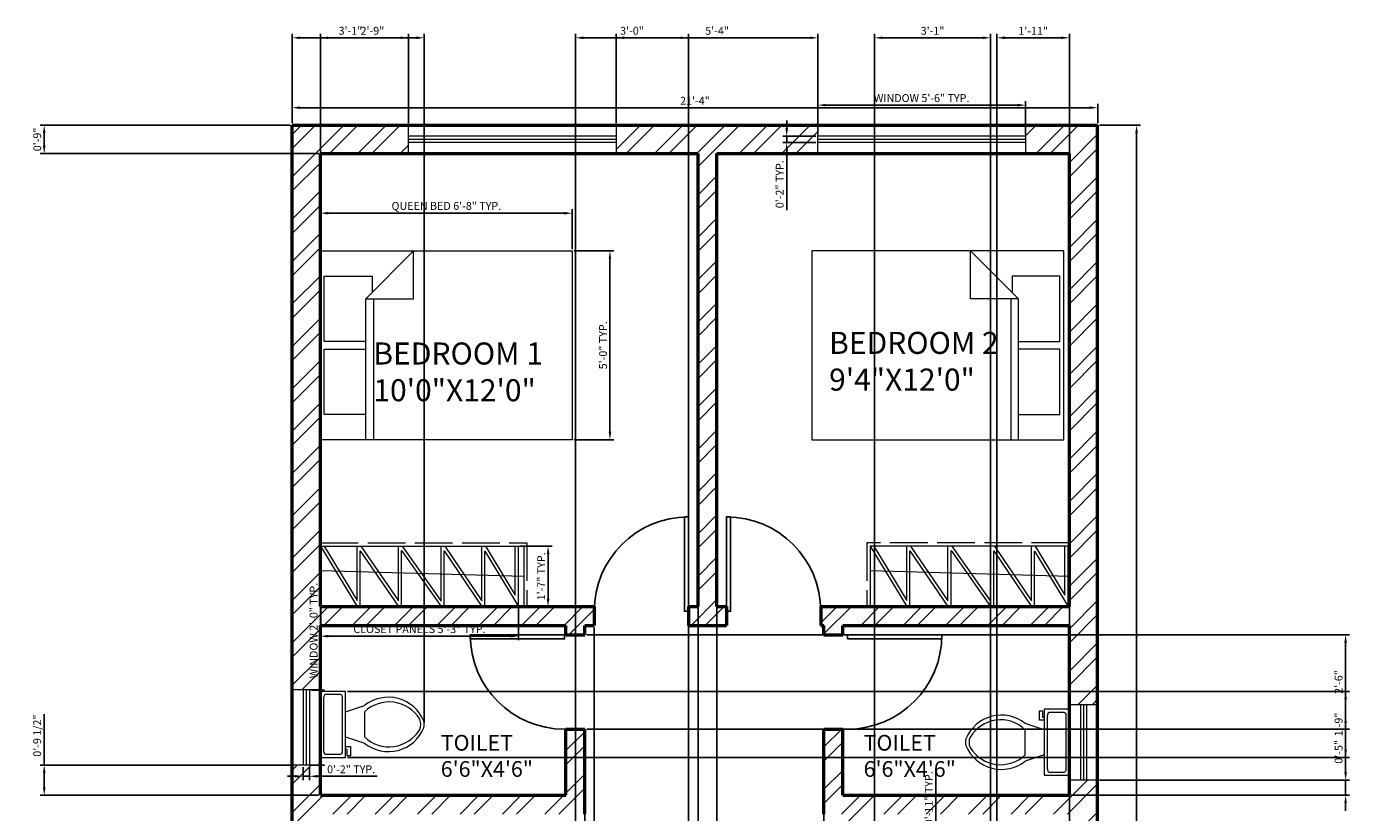
# Model space of a CAD drawing. Units: inches. Extents: x 1147 to 1568, y 1982 to 2559.
# Tile 4 of 4: x 1147 to 1568, y 2309 to 2559. Entities that reach past the tile are written whole.
import ezdxf

# ---------------------------------------------------------------- set-up
doc = ezdxf.new("R2010")
doc.units = ezdxf.units.IN
doc.linetypes.add('ACAD_ISO02W100', pattern=[15, 12, -3])
for name, color, linetype, lineweight in [('A-ANNO-DIMS', 2, 'Continuous', 18), ('A-DOOR', 4, 'Continuous', 25), ('A-FLOR-CASE', 8, 'Continuous', 18), ('A-FLOR-CASE-HIDN', 8, 'ACAD_ISO02W100', 18), ('A-FLOR-FIXT', 8, 'Continuous', 18), ('A-WALL', 7, 'Continuous', 50), ('A-WALL-PATT', 252, 'Continuous', 13)]:
    doc.layers.add(name, color=color, linetype=linetype, lineweight=lineweight)
for name, color, linetype, lineweight, true_color in [('A-AREA-IDEN', 244, 'Continuous', 25, 0x991b1e), ('A-FURN', 244, 'Continuous', 18, 0x991b1e), ('A-GLAZ', 177, 'Continuous', 18, 0x293189)]:
    doc.layers.add(name, color=color, linetype=linetype, lineweight=lineweight, true_color=true_color)
doc.styles.get("Standard").update_dxf_attribs({"font": 'arial.ttf'})
doc.dimstyles.new('ISO-25', dxfattribs={"dimtxt": 2.5, "dimasz": 2.5, "dimexe": 1.25, "dimexo": 0.625, "dimtad": 1, "dimlunit": 3, "dimtxsty": 'Standard', "dimcen": 2.5, "dimadec": 0, "dimazin": 0, "dimtfac": 1, "dimtmove": 0, "dimatfit": 3, "dimfxl": 1, "dimarcsym": 0})

# ---------------------------------------------------------------- blocks, each defined once
blk = doc.blocks.new('*U2')
for p, q in [((0, 0), (0, -6)), ((-40, 0), (-40, -6))]:
    blk.add_line(p, q)
blk.add_lwpolyline([(0, 0), (0, 40), (-1.75, 40), (-1.75, 0)], close=True)
blk.add_arc((0, 0), 40, 90, 180)
blk = doc.blocks.new('*U3')
for p, q in [((-40, 0), (-40, 6)), ((0, 0), (0, 6))]:
    blk.add_line(p, q)
blk.add_lwpolyline([(0, 0), (0, -40), (-1.75, -40), (-1.75, 0)], close=True)
blk.add_arc((0, 0), 40, 180, 270)
blk = doc.blocks.new('Bed - Queen')
for p, q in [((0, -80.00003), (0, 0)), ((0, 0), (59.99999, 0)), ((59.99999, 0), (59.99999, -80.00003)), ((7.99999, -1.2), (28.79998, -1.2)), ((7.99999, -14.4), (7.99999, -1.2)), ((28.79998, -1.2), (28.79998, -14.4)), ((31.19999, -1.2), (51.99999, -1.2)), ((31.19999, -14.4), (31.19999, -1.2)), ((51.99999, -1.2), (51.99999, -16.4)), ((0, -14.4), (44.8, -14.4)), ((44.8, -16.8), (0, -16.8)), ((59.99999, -29.6), (44.8, -14.4)), ((44.8, -14.4), (44.8, -29.6)), ((51.99999, -16.4), (46.79936, -16.4)), ((44.8, -29.6), (59.99999, -29.6)), ((59.99999, -80.00003), (0, -80.00003))]:
    blk.add_line(p, q)
blk = doc.blocks.new('*U6')
for p, q in [((9.5, -6), (9.5, -2)), ((-8, -8.5), (-8, -8)), ((-7, -8), (-7, -9.5)), ((-4, -8), (-6, -14)), ((4, -8), (6, -14)), ((-10, -8.5), (-8, -8.5)), ((-10, -9.5), (-10, -8.5)), ((-7, -9.5), (-10, -9.5)), ((4, -14), (-4, -14))]:
    blk.add_line(p, q)
blk.add_lwpolyline([(10.5, -8), (10.5, 0), (-10.5, 0), (-10.5, -8)], close=True)
for points in [[(-9.5, -2), (-9.5, -6)], [(8.5, -1), (-8.5, -1)], [(-8.5, -7), (8.5, -7)]]:
    blk.add_lwpolyline(points)
for centre, radius, start, end in [((-8.62, -1.88), 0.884, 81.8699, 188.1301), ((8.62, -1.88), 0.884, 351.8699, 98.1301), ((-8.62, -6.12), 0.884, 171.8699, 278.1301), ((8.62, -6.12), 0.884, 261.8699, 8.1301), ((3.52, -21.58), 12.17, 141.4691, 247.9714), ((4.2, -21.82), 11.33, 136.3677, 238.9468), ((-3.52, -21.58), 12.17, 292.0284, 38.5307), ((-4.2, -21.82), 11.33, 301.053, 43.6321), ((0, -27.88), 4, 245.7318, 294.2682), ((0, -29), 4, 254.8605, 285.1395)]:
    blk.add_arc(centre, radius, start, end)
blk = doc.blocks.new('*D13')
at = {"layer": 'A-ANNO-DIMS', "color": 0, "lineweight": -2, "transparency": 16777216}
for p, q in [((1488.23, 2527.7), (1501.22, 2527.7)), ((1499.97, 2525.2), (1499.97, 2020.2)), ((1488.23, 2017.7), (1501.22, 2017.7))]:
    blk.add_line(p, q, dxfattribs=at)
at = {"layer": 'A-ANNO-DIMS', "color": 0, "transparency": 16777216}
for points in [[(1499.56, 2525.2), (1500.39, 2525.2), (1499.97, 2527.7)], [(1499.56, 2020.2), (1500.39, 2020.2), (1499.97, 2017.7)]]:
    blk.add_solid(points, dxfattribs=at)
at = {"layer": 'Defpoints', "color": 0, "transparency": 16777216}
for p in [(1487.61, 2527.7), (1487.61, 2017.7), (1499.97, 2017.7)]:
    blk.add_point(p, dxfattribs=at)
at = {"layer": 'A-ANNO-DIMS', "color": 0, "transparency": 16777216, "insert": (1498.07, 2272.7), "char_height": 2.5, "attachment_point": 5, "rotation": 90}
blk.add_mtext('42\'-6"', dxfattribs=at)
blk = doc.blocks.new('*D14')
at = {"layer": 'A-ANNO-DIMS', "color": 0, "lineweight": -2, "transparency": 16777216}
for p, q in [((1231.61, 2528.33), (1231.61, 2534.54)), ((1485.11, 2533.29), (1234.11, 2533.29)), ((1487.61, 2528.33), (1487.61, 2534.54))]:
    blk.add_line(p, q, dxfattribs=at)
at = {"layer": 'A-ANNO-DIMS', "color": 0, "transparency": 16777216}
for points in [[(1234.11, 2533.7), (1234.11, 2532.87), (1231.61, 2533.29)], [(1485.11, 2533.7), (1485.11, 2532.87), (1487.61, 2533.29)]]:
    blk.add_solid(points, dxfattribs=at)
at = {"layer": 'Defpoints', "color": 0, "transparency": 16777216}
for p in [(1231.61, 2533.29), (1231.61, 2527.7), (1487.61, 2527.7)]:
    blk.add_point(p, dxfattribs=at)
at = {"layer": 'A-ANNO-DIMS', "color": 0, "transparency": 16777216, "insert": (1359.61, 2535.17), "char_height": 2.5, "attachment_point": 5}
blk.add_mtext('21\'-4"', dxfattribs=at)
blk = doc.blocks.new('WIN-GLAZ-66IN')
for p, q in [((0, 2), (66, 2)), ((0, 1), (66, 1)), ((0, 0), (66, 0))]:
    blk.add_line(p, q)
blk = doc.blocks.new('WIN-GLAZ-24IN')
for p, q in [((0, 23.82), (0, 0)), ((1, 23.82), (1, 0)), ((2, 23.82), (2, 0))]:
    blk.add_line(p, q)
blk = doc.blocks.new('CLOSET-PANEL-SET')
for p, q in [((0, 19.2), (11.64, 0)), ((1.17, 19.2), (11.64, 1.93)), ((11.64, 1.93), (11.64, 19.2)), ((12.64, 17.74), (24.75, 0)), ((12.64, 0), (12.64, 17.74)), ((12.85, 19.2), (24.75, 1.77)), ((24.75, 1.77), (24.75, 19.2)), ((25.75, 17.78), (38.31, 0)), ((25.75, 0), (25.75, 17.78)), ((25.98, 19.2), (38.31, 1.73)), ((38.31, 1.73), (38.31, 19.2)), ((39.31, 17.72), (51.27, 0)), ((39.31, 0), (39.31, 17.72)), ((39.52, 19.2), (51.27, 1.79)), ((51.27, 1.79), (51.27, 19.2)), ((52.27, 17.55), (62.9, 0)), ((52.27, 0), (52.27, 17.55)), ((52.44, 19.2), (61.9, 3.58)), ((61.9, 3.58), (61.9, 19.2)), ((62.9, 0), (62.9, 19.2))]:
    blk.add_line(p, q)
blk = doc.blocks.new('*D21')
at = {"layer": 'A-ANNO-DIMS', "color": 0, "lineweight": -2, "transparency": 16777216}
for p, q in [((1398.68, 2524.83), (1398.68, 2535.35)), ((1462.18, 2534.1), (1401.18, 2534.1)), ((1464.68, 2524.83), (1464.68, 2535.35))]:
    blk.add_line(p, q, dxfattribs=at)
at = {"layer": 'A-ANNO-DIMS', "color": 0, "transparency": 16777216}
for points in [[(1401.18, 2534.52), (1401.18, 2533.69), (1398.68, 2534.1)], [(1462.18, 2534.52), (1462.18, 2533.69), (1464.68, 2534.1)]]:
    blk.add_solid(points, dxfattribs=at)
at = {"layer": 'Defpoints', "color": 0, "transparency": 16777216}
for p in [(1398.68, 2534.1), (1398.68, 2524.2), (1464.68, 2524.2)]:
    blk.add_point(p, dxfattribs=at)
at = {"layer": 'A-ANNO-DIMS', "color": 0, "transparency": 16777216, "insert": (1431.68, 2536.02), "char_height": 2.5, "attachment_point": 5}
blk.add_mtext('WINDOW 5\'-6" TYP.', dxfattribs=at)
blk = doc.blocks.new('*D22')
at = {"layer": 'A-ANNO-DIMS', "color": 0, "lineweight": -2, "transparency": 16777216}
for p, q in [((1388.78, 2526.7), (1388.78, 2529.2)), ((1398.05, 2524.2), (1387.53, 2524.2)), ((1388.78, 2524.2), (1388.78, 2522.2)), ((1398.05, 2522.2), (1387.53, 2522.2)), ((1388.78, 2519.7), (1388.78, 2500.72))]:
    blk.add_line(p, q, dxfattribs=at)
at = {"layer": 'A-ANNO-DIMS', "color": 0, "transparency": 16777216}
for points in [[(1388.36, 2526.7), (1389.2, 2526.7), (1388.78, 2524.2)], [(1388.36, 2519.7), (1389.2, 2519.7), (1388.78, 2522.2)]]:
    blk.add_solid(points, dxfattribs=at)
at = {"layer": 'Defpoints', "color": 0, "transparency": 16777216}
for p in [(1398.68, 2524.2), (1388.78, 2522.2), (1398.68, 2522.2)]:
    blk.add_point(p, dxfattribs=at)
at = {"layer": 'A-ANNO-DIMS', "color": 0, "transparency": 16777216, "insert": (1386.88, 2508.96), "char_height": 2.5, "attachment_point": 5, "rotation": 90}
blk.add_mtext('0\'-2" TYP.', dxfattribs=at)
blk = doc.blocks.new('*D23')
at = {"layer": 'A-ANNO-DIMS', "color": 0, "lineweight": -2, "transparency": 16777216}
for p, q in [((1240.68, 2348.11), (1240.68, 2383.5)), ((1237.73, 2348.11), (1241.93, 2348.11)), ((1240.68, 2326.8), (1240.68, 2345.61)), ((1237.73, 2324.3), (1241.93, 2324.3))]:
    blk.add_line(p, q, dxfattribs=at)
at = {"layer": 'A-ANNO-DIMS', "color": 0, "transparency": 16777216}
for points in [[(1240.26, 2345.61), (1241.1, 2345.61), (1240.68, 2348.11)], [(1240.26, 2326.8), (1241.1, 2326.8), (1240.68, 2324.3)]]:
    blk.add_solid(points, dxfattribs=at)
at = {"layer": 'Defpoints', "color": 0, "transparency": 16777216}
for p in [(1237.11, 2348.11), (1240.68, 2348.11), (1237.11, 2324.3)]:
    blk.add_point(p, dxfattribs=at)
at = {"layer": 'A-ANNO-DIMS', "color": 0, "transparency": 16777216, "insert": (1238.76, 2367.06), "char_height": 2.5, "attachment_point": 5, "rotation": 90}
blk.add_mtext('WINDOW 2\'-0" TYP.', dxfattribs=at)
blk = doc.blocks.new('*D24')
at = {"layer": 'A-ANNO-DIMS', "color": 0, "lineweight": -2, "transparency": 16777216}
for p, q in [((1235.11, 2323.67), (1235.11, 2319.47)), ((1237.11, 2323.67), (1237.11, 2319.47)), ((1232.61, 2320.72), (1230.11, 2320.72)), ((1235.11, 2320.72), (1237.11, 2320.72)), ((1239.61, 2320.72), (1258.6, 2320.72))]:
    blk.add_line(p, q, dxfattribs=at)
at = {"layer": 'A-ANNO-DIMS', "color": 0, "transparency": 16777216}
for points in [[(1232.61, 2321.14), (1232.61, 2320.31), (1235.11, 2320.72)], [(1239.61, 2321.14), (1239.61, 2320.31), (1237.11, 2320.72)]]:
    blk.add_solid(points, dxfattribs=at)
at = {"layer": 'Defpoints', "color": 0, "transparency": 16777216}
for p in [(1235.11, 2324.3), (1237.11, 2324.3), (1237.11, 2320.72)]:
    blk.add_point(p, dxfattribs=at)
at = {"layer": 'A-ANNO-DIMS', "color": 0, "transparency": 16777216, "insert": (1250.35, 2322.62), "char_height": 2.5, "attachment_point": 5}
blk.add_mtext('0\'-2" TYP.', dxfattribs=at)
blk = doc.blocks.new('*D27')
at = {"layer": 'A-ANNO-DIMS', "color": 0, "lineweight": -2, "transparency": 16777216}
for p, q in [((1240.61, 2488.36), (1240.61, 2500.99)), ((1318.11, 2499.74), (1243.11, 2499.74)), ((1320.61, 2488.36), (1320.61, 2500.99))]:
    blk.add_line(p, q, dxfattribs=at)
at = {"layer": 'A-ANNO-DIMS', "color": 0, "transparency": 16777216}
for points in [[(1243.11, 2500.16), (1243.11, 2499.32), (1240.61, 2499.74)], [(1318.11, 2500.16), (1318.11, 2499.32), (1320.61, 2499.74)]]:
    blk.add_solid(points, dxfattribs=at)
at = {"layer": 'Defpoints', "color": 0, "transparency": 16777216}
for p in [(1240.61, 2499.74), (1240.61, 2487.74), (1320.61, 2487.74)]:
    blk.add_point(p, dxfattribs=at)
at = {"layer": 'A-ANNO-DIMS', "color": 0, "transparency": 16777216, "insert": (1280.61, 2501.73), "char_height": 2.5, "attachment_point": 5}
blk.add_mtext('QUEEN BED 6\'-8" TYP.', dxfattribs=at)
blk = doc.blocks.new('*D28')
at = {"layer": 'A-ANNO-DIMS', "color": 0, "lineweight": -2, "transparency": 16777216}
for p, q in [((1321.23, 2487.74), (1333.86, 2487.74)), ((1332.61, 2430.24), (1332.61, 2485.24)), ((1321.23, 2427.74), (1333.86, 2427.74))]:
    blk.add_line(p, q, dxfattribs=at)
at = {"layer": 'A-ANNO-DIMS', "color": 0, "transparency": 16777216}
for points in [[(1332.19, 2485.24), (1333.02, 2485.24), (1332.61, 2487.74)], [(1332.19, 2430.24), (1333.02, 2430.24), (1332.61, 2427.74)]]:
    blk.add_solid(points, dxfattribs=at)
at = {"layer": 'Defpoints', "color": 0, "transparency": 16777216}
for p in [(1320.61, 2487.74), (1332.61, 2487.74), (1320.61, 2427.74)]:
    blk.add_point(p, dxfattribs=at)
at = {"layer": 'A-ANNO-DIMS', "color": 0, "transparency": 16777216, "insert": (1330.71, 2457.74), "char_height": 2.5, "attachment_point": 5, "rotation": 90}
blk.add_mtext('5\'-0" TYP.', dxfattribs=at)
blk = doc.blocks.new('*D32')
at = {"layer": 'A-ANNO-DIMS', "color": 0, "lineweight": -2, "transparency": 16777216}
for p, q in [((1436.16, 2302.04), (1436.16, 2322.97)), ((1434.67, 2302.04), (1437.41, 2302.04)), ((1436.16, 2293.51), (1436.16, 2299.54)), ((1434.67, 2291.01), (1437.41, 2291.01))]:
    blk.add_line(p, q, dxfattribs=at)
at = {"layer": 'A-ANNO-DIMS', "color": 0, "transparency": 16777216}
for points in [[(1435.75, 2299.54), (1436.58, 2299.54), (1436.16, 2302.04)], [(1435.75, 2293.51), (1436.58, 2293.51), (1436.16, 2291.01)]]:
    blk.add_solid(points, dxfattribs=at)
at = {"layer": 'Defpoints', "color": 0, "transparency": 16777216}
for p in [(1434.04, 2302.04), (1436.16, 2302.04), (1434.04, 2291.01)]:
    blk.add_point(p, dxfattribs=at)
at = {"layer": 'A-ANNO-DIMS', "color": 0, "transparency": 16777216, "insert": (1434.26, 2313.75), "char_height": 2.5, "attachment_point": 5, "rotation": 90}
blk.add_mtext('0\'-11" TYP.', dxfattribs=at)
blk = doc.blocks.new('*D33')
at = {"layer": 'A-ANNO-DIMS', "color": 0, "lineweight": -2, "transparency": 16777216}
for p, q in [((1240.61, 2374.08), (1240.61, 2364.02)), ((1303.5, 2374.08), (1303.5, 2364.02)), ((1243.11, 2365.27), (1301, 2365.27))]:
    blk.add_line(p, q, dxfattribs=at)
at = {"layer": 'A-ANNO-DIMS', "color": 0, "transparency": 16777216}
for points in [[(1243.11, 2365.69), (1243.11, 2364.85), (1240.61, 2365.27)], [(1301, 2365.69), (1301, 2364.85), (1303.5, 2365.27)]]:
    blk.add_solid(points, dxfattribs=at)
at = {"layer": 'Defpoints', "color": 0, "transparency": 16777216}
for p in [(1240.61, 2374.7), (1303.5, 2374.7), (1303.5, 2365.27)]:
    blk.add_point(p, dxfattribs=at)
at = {"layer": 'A-ANNO-DIMS', "color": 0, "transparency": 16777216, "insert": (1272.06, 2367.19), "char_height": 2.5, "attachment_point": 5}
blk.add_mtext('CLOSET PANELS 5\'-3" TYP.', dxfattribs=at)
blk = doc.blocks.new('*D34')
at = {"layer": 'A-ANNO-DIMS', "color": 0, "lineweight": -2, "transparency": 16777216}
for p, q in [((1304.13, 2393.9), (1314.19, 2393.9)), ((1312.94, 2377.2), (1312.94, 2391.4)), ((1304.13, 2374.7), (1314.19, 2374.7))]:
    blk.add_line(p, q, dxfattribs=at)
at = {"layer": 'A-ANNO-DIMS', "color": 0, "transparency": 16777216}
for points in [[(1312.52, 2391.4), (1313.36, 2391.4), (1312.94, 2393.9)], [(1312.52, 2377.2), (1313.36, 2377.2), (1312.94, 2374.7)]]:
    blk.add_solid(points, dxfattribs=at)
at = {"layer": 'Defpoints', "color": 0, "transparency": 16777216}
for p in [(1303.5, 2393.9), (1312.94, 2393.9), (1303.5, 2374.7)]:
    blk.add_point(p, dxfattribs=at)
at = {"layer": 'A-ANNO-DIMS', "color": 0, "transparency": 16777216, "insert": (1311.06, 2384.3), "char_height": 2.5, "attachment_point": 5, "rotation": 90}
blk.add_mtext('1\'-7" TYP.', dxfattribs=at)
blk = doc.blocks.new('*D43')
at = {"layer": 'A-ANNO-DIMS', "color": 0, "lineweight": -2, "transparency": 16777216}
for p, q in [((1327.61, 2368.08), (1327.61, 1981.52)), ((1357.61, 2368.08), (1357.61, 1981.52)), ((1330.11, 1982.77), (1355.11, 1982.77))]:
    blk.add_line(p, q, dxfattribs=at)
at = {"layer": 'A-ANNO-DIMS', "color": 0, "transparency": 16777216}
for points in [[(1330.11, 1983.19), (1330.11, 1982.35), (1327.61, 1982.77)], [(1355.11, 1983.19), (1355.11, 1982.35), (1357.61, 1982.77)]]:
    blk.add_solid(points, dxfattribs=at)
at = {"layer": 'Defpoints', "color": 0, "transparency": 16777216}
for p in [(1327.61, 2368.7), (1357.61, 2368.7), (1357.61, 1982.77)]:
    blk.add_point(p, dxfattribs=at)
at = {"layer": 'A-ANNO-DIMS', "color": 0, "transparency": 16777216, "insert": (1342.61, 1984.67), "char_height": 2.5, "attachment_point": 5}
blk.add_mtext('2\'-6"', dxfattribs=at)
blk = doc.blocks.new('*D44')
at = {"layer": 'A-ANNO-DIMS', "color": 0, "lineweight": -2, "transparency": 16777216}
for p, q in [((1325.23, 2365.7), (1567.66, 2365.7)), ((1566.41, 2338.2), (1566.41, 2363.2)), ((1325.23, 2335.7), (1567.66, 2335.7))]:
    blk.add_line(p, q, dxfattribs=at)
at = {"layer": 'A-ANNO-DIMS', "color": 0, "transparency": 16777216}
for points in [[(1565.99, 2363.2), (1566.82, 2363.2), (1566.41, 2365.7)], [(1565.99, 2338.2), (1566.82, 2338.2), (1566.41, 2335.7)]]:
    blk.add_solid(points, dxfattribs=at)
at = {"layer": 'Defpoints', "color": 0, "transparency": 16777216}
for p in [(1324.61, 2365.7), (1566.41, 2365.7), (1324.61, 2335.7)]:
    blk.add_point(p, dxfattribs=at)
at = {"layer": 'A-ANNO-DIMS', "color": 0, "transparency": 16777216, "insert": (1564.51, 2350.7), "char_height": 2.5, "attachment_point": 5, "rotation": 90}
blk.add_mtext('2\'-6"', dxfattribs=at)
blk = doc.blocks.new('*D45')
at = {"layer": 'A-ANNO-DIMS', "color": 0, "lineweight": -2, "transparency": 16777216}
for p, q in [((1321.61, 2177.33), (1321.61, 2556.75)), ((1357.61, 2177.33), (1357.61, 2556.75)), ((1324.11, 2555.5), (1355.11, 2555.5))]:
    blk.add_line(p, q, dxfattribs=at)
at = {"layer": 'A-ANNO-DIMS', "color": 0, "transparency": 16777216}
for points in [[(1324.11, 2555.92), (1324.11, 2555.09), (1321.61, 2555.5)], [(1355.11, 2555.92), (1355.11, 2555.09), (1357.61, 2555.5)]]:
    blk.add_solid(points, dxfattribs=at)
at = {"layer": 'Defpoints', "color": 0, "transparency": 16777216}
for p in [(1357.61, 2555.5), (1321.61, 2176.7), (1357.61, 2176.7)]:
    blk.add_point(p, dxfattribs=at)
at = {"layer": 'A-ANNO-DIMS', "color": 0, "transparency": 16777216, "insert": (1339.61, 2557.41), "char_height": 2.5, "attachment_point": 5}
blk.add_mtext('3\'-0"', dxfattribs=at)
blk = doc.blocks.new('*D51')
at = {"layer": 'A-ANNO-DIMS', "color": 0, "lineweight": -2, "transparency": 16777216}
for p, q in [((1360.61, 2518.08), (1360.61, 1981.52)), ((1366.61, 2518.08), (1366.61, 1981.52)), ((1358.11, 1982.77), (1355.61, 1982.77)), ((1360.61, 1982.77), (1366.61, 1982.77)), ((1369.11, 1982.77), (1379.5, 1982.77))]:
    blk.add_line(p, q, dxfattribs=at)
at = {"layer": 'A-ANNO-DIMS', "color": 0, "transparency": 16777216}
for points in [[(1358.11, 1983.19), (1358.11, 1982.35), (1360.61, 1982.77)], [(1369.11, 1983.19), (1369.11, 1982.35), (1366.61, 1982.77)]]:
    blk.add_solid(points, dxfattribs=at)
at = {"layer": 'Defpoints', "color": 0, "transparency": 16777216}
for p in [(1360.61, 2518.7), (1366.61, 2518.7), (1366.61, 1982.77)]:
    blk.add_point(p, dxfattribs=at)
at = {"layer": 'A-ANNO-DIMS', "color": 0, "transparency": 16777216, "insert": (1375.55, 1984.67), "char_height": 2.5, "attachment_point": 5}
blk.add_mtext('0\'-6"', dxfattribs=at)
blk = doc.blocks.new('*D52')
at = {"layer": 'A-ANNO-DIMS', "color": 0, "lineweight": -2, "transparency": 16777216}
for p, q in [((1231.61, 2528.33), (1231.61, 2556.75)), ((1268.63, 2528.33), (1268.63, 2556.75)), ((1234.11, 2555.5), (1266.13, 2555.5))]:
    blk.add_line(p, q, dxfattribs=at)
at = {"layer": 'A-ANNO-DIMS', "color": 0, "transparency": 16777216}
for points in [[(1234.11, 2555.92), (1234.11, 2555.09), (1231.61, 2555.5)], [(1266.13, 2555.92), (1266.13, 2555.09), (1268.63, 2555.5)]]:
    blk.add_solid(points, dxfattribs=at)
at = {"layer": 'Defpoints', "color": 0, "transparency": 16777216}
for p in [(1268.63, 2555.5), (1231.61, 2527.7), (1268.63, 2527.7)]:
    blk.add_point(p, dxfattribs=at)
at = {"layer": 'A-ANNO-DIMS', "color": 0, "transparency": 16777216, "insert": (1250.12, 2557.41), "char_height": 2.5, "attachment_point": 5}
blk.add_mtext('3\'-1"', dxfattribs=at)
blk = doc.blocks.new('*D53')
at = {"layer": 'A-ANNO-DIMS', "color": 0, "lineweight": -2, "transparency": 16777216}
for p, q in [((1334.63, 2528.33), (1334.63, 2556.75)), ((1398.68, 2528.33), (1398.68, 2556.75)), ((1337.13, 2555.5), (1396.18, 2555.5))]:
    blk.add_line(p, q, dxfattribs=at)
at = {"layer": 'A-ANNO-DIMS', "color": 0, "transparency": 16777216}
for points in [[(1337.13, 2555.92), (1337.13, 2555.09), (1334.63, 2555.5)], [(1396.18, 2555.92), (1396.18, 2555.09), (1398.68, 2555.5)]]:
    blk.add_solid(points, dxfattribs=at)
at = {"layer": 'Defpoints', "color": 0, "transparency": 16777216}
for p in [(1398.68, 2555.5), (1334.63, 2527.7), (1398.68, 2527.7)]:
    blk.add_point(p, dxfattribs=at)
at = {"layer": 'A-ANNO-DIMS', "color": 0, "transparency": 16777216, "insert": (1366.65, 2557.4), "char_height": 2.5, "attachment_point": 5}
blk.add_mtext('5\'-4"', dxfattribs=at)
blk = doc.blocks.new('*D54')
at = {"layer": 'A-ANNO-DIMS', "color": 0, "lineweight": -2, "transparency": 16777216}
for p, q in [((1230.98, 2527.7), (1151.56, 2527.7)), ((1152.81, 2525.2), (1152.81, 2521.2)), ((1239.98, 2518.7), (1151.56, 2518.7))]:
    blk.add_line(p, q, dxfattribs=at)
at = {"layer": 'A-ANNO-DIMS', "color": 0, "transparency": 16777216}
for points in [[(1152.39, 2525.2), (1153.22, 2525.2), (1152.81, 2527.7)], [(1152.39, 2521.2), (1153.22, 2521.2), (1152.81, 2518.7)]]:
    blk.add_solid(points, dxfattribs=at)
at = {"layer": 'Defpoints', "color": 0, "transparency": 16777216}
for p in [(1231.61, 2527.7), (1152.81, 2518.7), (1240.61, 2518.7)]:
    blk.add_point(p, dxfattribs=at)
at = {"layer": 'A-ANNO-DIMS', "color": 0, "transparency": 16777216, "insert": (1150.91, 2523.2), "char_height": 2.5, "attachment_point": 5, "rotation": 90}
blk.add_mtext('0\'-9"', dxfattribs=at)
blk = doc.blocks.new('*D58')
at = {"layer": 'A-ANNO-DIMS', "color": 0, "lineweight": -2, "transparency": 16777216}
for p, q in [((1152.81, 2324.3), (1152.81, 2340.52)), ((1230.98, 2324.3), (1151.56, 2324.3)), ((1152.81, 2317.2), (1152.81, 2321.8)), ((1239.98, 2314.7), (1151.56, 2314.7))]:
    blk.add_line(p, q, dxfattribs=at)
at = {"layer": 'A-ANNO-DIMS', "color": 0, "transparency": 16777216}
for points in [[(1152.39, 2321.8), (1153.22, 2321.8), (1152.81, 2324.3)], [(1152.39, 2317.2), (1153.22, 2317.2), (1152.81, 2314.7)]]:
    blk.add_solid(points, dxfattribs=at)
at = {"layer": 'Defpoints', "color": 0, "transparency": 16777216}
for p in [(1152.81, 2324.3), (1231.61, 2324.3), (1240.61, 2314.7)]:
    blk.add_point(p, dxfattribs=at)
at = {"layer": 'A-ANNO-DIMS', "color": 0, "transparency": 16777216, "insert": (1150.89, 2333.66), "char_height": 2.5, "attachment_point": 5, "rotation": 90}
blk.add_mtext('0\'-9 1/2"', dxfattribs=at)
blk = doc.blocks.new('*D59')
at = {"layer": 'A-ANNO-DIMS', "color": 0, "lineweight": -2, "transparency": 16777216}
for p, q in [((1566.41, 2322.05), (1566.41, 2332.44)), ((1488.23, 2319.55), (1567.66, 2319.55)), ((1566.41, 2314.7), (1566.41, 2319.55)), ((1479.23, 2314.7), (1567.66, 2314.7)), ((1566.41, 2312.2), (1566.41, 2309.7))]:
    blk.add_line(p, q, dxfattribs=at)
at = {"layer": 'A-ANNO-DIMS', "color": 0, "transparency": 16777216}
for points in [[(1565.99, 2322.05), (1566.82, 2322.05), (1566.41, 2319.55)], [(1565.99, 2312.2), (1566.82, 2312.2), (1566.41, 2314.7)]]:
    blk.add_solid(points, dxfattribs=at)
at = {"layer": 'Defpoints', "color": 0, "transparency": 16777216}
for p in [(1487.61, 2319.55), (1566.41, 2319.55), (1478.61, 2314.7)]:
    blk.add_point(p, dxfattribs=at)
at = {"layer": 'A-ANNO-DIMS', "color": 0, "transparency": 16777216, "insert": (1564.51, 2328.5), "char_height": 2.5, "attachment_point": 5, "rotation": 90}
blk.add_mtext('0\'-5"', dxfattribs=at)
blk = doc.blocks.new('*D61')
at = {"layer": 'A-ANNO-DIMS', "color": 0, "lineweight": -2, "transparency": 16777216}
for p, q in [((1455.61, 2213.33), (1455.61, 2556.75)), ((1478.61, 2213.33), (1478.61, 2556.75)), ((1458.11, 2555.5), (1476.11, 2555.5))]:
    blk.add_line(p, q, dxfattribs=at)
at = {"layer": 'A-ANNO-DIMS', "color": 0, "transparency": 16777216}
for points in [[(1458.11, 2555.92), (1458.11, 2555.09), (1455.61, 2555.5)], [(1476.11, 2555.92), (1476.11, 2555.09), (1478.61, 2555.5)]]:
    blk.add_solid(points, dxfattribs=at)
at = {"layer": 'Defpoints', "color": 0, "transparency": 16777216}
for p in [(1478.61, 2555.5), (1455.61, 2212.7), (1478.61, 2212.7)]:
    blk.add_point(p, dxfattribs=at)
at = {"layer": 'A-ANNO-DIMS', "color": 0, "transparency": 16777216, "insert": (1467.11, 2557.38), "char_height": 2.5, "attachment_point": 5}
blk.add_mtext('1\'-11"', dxfattribs=at)
blk = doc.blocks.new('*D62')
at = {"layer": 'A-ANNO-DIMS', "color": 0, "lineweight": -2, "transparency": 16777216}
for p, q in [((1324.61, 2335.08), (1324.61, 1981.52)), ((1400.61, 2335.08), (1400.61, 1981.52)), ((1327.11, 1982.77), (1398.11, 1982.77))]:
    blk.add_line(p, q, dxfattribs=at)
at = {"layer": 'A-ANNO-DIMS', "color": 0, "transparency": 16777216}
for points in [[(1327.11, 1983.19), (1327.11, 1982.35), (1324.61, 1982.77)], [(1398.11, 1983.19), (1398.11, 1982.35), (1400.61, 1982.77)]]:
    blk.add_solid(points, dxfattribs=at)
at = {"layer": 'Defpoints', "color": 0, "transparency": 16777216}
for p in [(1324.61, 2335.7), (1400.61, 2335.7), (1400.61, 1982.77)]:
    blk.add_point(p, dxfattribs=at)
at = {"layer": 'A-ANNO-DIMS', "color": 0, "transparency": 16777216, "insert": (1362.61, 1984.67), "char_height": 2.5, "attachment_point": 5}
blk.add_mtext('6\'-4"', dxfattribs=at)
blk = doc.blocks.new('*D63')
at = {"layer": 'A-ANNO-DIMS', "color": 0, "lineweight": -2, "transparency": 16777216}
for p, q in [((1240.61, 2348.35), (1240.61, 2556.75)), ((1273.61, 2337.85), (1273.61, 2556.75)), ((1243.11, 2555.5), (1271.11, 2555.5))]:
    blk.add_line(p, q, dxfattribs=at)
at = {"layer": 'A-ANNO-DIMS', "color": 0, "transparency": 16777216}
for points in [[(1243.11, 2555.92), (1243.11, 2555.09), (1240.61, 2555.5)], [(1271.11, 2555.92), (1271.11, 2555.09), (1273.61, 2555.5)]]:
    blk.add_solid(points, dxfattribs=at)
at = {"layer": 'Defpoints', "color": 0, "transparency": 16777216}
for p in [(1273.61, 2555.5), (1240.61, 2347.72), (1273.61, 2337.22)]:
    blk.add_point(p, dxfattribs=at)
at = {"layer": 'A-ANNO-DIMS', "color": 0, "transparency": 16777216, "insert": (1257.11, 2557.41), "char_height": 2.5, "attachment_point": 5}
blk.add_mtext('2\'-9"', dxfattribs=at)
blk = doc.blocks.new('*D64')
at = {"layer": 'A-ANNO-DIMS', "color": 0, "lineweight": -2, "transparency": 16777216}
for p, q in [((1249.23, 2347.72), (1567.66, 2347.72)), ((1566.41, 2329.22), (1566.41, 2345.22)), ((1249.23, 2326.72), (1567.66, 2326.72))]:
    blk.add_line(p, q, dxfattribs=at)
at = {"layer": 'A-ANNO-DIMS', "color": 0, "transparency": 16777216}
for points in [[(1565.99, 2345.22), (1566.82, 2345.22), (1566.41, 2347.72)], [(1565.99, 2329.22), (1566.82, 2329.22), (1566.41, 2326.72)]]:
    blk.add_solid(points, dxfattribs=at)
at = {"layer": 'Defpoints', "color": 0, "transparency": 16777216}
for p in [(1248.61, 2347.72), (1566.41, 2347.72), (1248.61, 2326.72)]:
    blk.add_point(p, dxfattribs=at)
at = {"layer": 'A-ANNO-DIMS', "color": 0, "transparency": 16777216, "insert": (1564.51, 2337.22), "char_height": 2.5, "attachment_point": 5, "rotation": 90}
blk.add_mtext('1\'-9"', dxfattribs=at)
blk = doc.blocks.new('*D67')
at = {"layer": 'A-ANNO-DIMS', "color": 0, "lineweight": -2, "transparency": 16777216}
for p, q in [((1416.72, 2305.68), (1416.72, 2556.75)), ((1453.56, 2305.68), (1453.56, 2556.75)), ((1419.22, 2555.5), (1451.06, 2555.5))]:
    blk.add_line(p, q, dxfattribs=at)
at = {"layer": 'A-ANNO-DIMS', "color": 0, "transparency": 16777216}
for points in [[(1419.22, 2555.92), (1419.22, 2555.09), (1416.72, 2555.5)], [(1451.06, 2555.92), (1451.06, 2555.09), (1453.56, 2555.5)]]:
    blk.add_solid(points, dxfattribs=at)
at = {"layer": 'Defpoints', "color": 0, "transparency": 16777216}
for p in [(1453.56, 2555.5), (1416.72, 2305.06), (1453.56, 2305.06)]:
    blk.add_point(p, dxfattribs=at)
at = {"layer": 'A-ANNO-DIMS', "color": 0, "transparency": 16777216, "insert": (1435.14, 2557.41), "char_height": 2.5, "attachment_point": 5}
blk.add_mtext('3\'-1"', dxfattribs=at)

msp = doc.modelspace()

# ---------------------------------------------------------------- hatches: boundary and pattern name
at = {"layer": 'A-WALL-PATT'}
h = msp.add_hatch(dxfattribs=at)
h.set_pattern_fill('ANSI32', color=256)
h.paths.add_polyline_path([(1240.607, 2518.704), (1268.63, 2518.704), (1268.63, 2527.704), (1231.607, 2527.704), (1231.607, 2348.295), (1240.607, 2348.295), (1240.607, 2368.704), (1318.607, 2368.704), (1318.607, 2365.704), (1324.607, 2365.704), (1324.607, 2368.704), (1327.607, 2368.704), (1327.607, 2374.704), (1240.607, 2374.704)])
h.paths.add_polyline_path([(1324.607, 2335.704), (1318.607, 2335.704), (1318.607, 2314.704), (1240.607, 2314.704), (1240.607, 2324.295), (1231.607, 2324.295), (1231.607, 2247.419), (1240.607, 2247.419), (1240.607, 2308.704), (1324.607, 2308.704)])
h.paths.add_polyline_path([(1487.607, 2527.704), (1464.679, 2527.704), (1464.679, 2518.704), (1478.607, 2518.704), (1478.607, 2374.704), (1399.607, 2374.704), (1399.607, 2368.704), (1400.607, 2368.704), (1400.607, 2365.704), (1406.607, 2365.704), (1406.607, 2368.704), (1478.607, 2368.704), (1478.607, 2343.549), (1487.607, 2343.549)])
h.paths.add_polyline_path([(1366.607, 2518.704), (1398.679, 2518.704), (1398.679, 2527.704), (1334.63, 2527.704), (1334.63, 2518.704), (1360.607, 2518.704), (1360.607, 2374.704), (1357.607, 2374.704), (1357.607, 2368.704), (1369.607, 2368.704), (1369.607, 2374.704), (1366.607, 2374.704)])
h.paths.add_polyline_path([(1487.607, 2319.549), (1478.607, 2319.549), (1478.607, 2314.704), (1406.607, 2314.704), (1406.607, 2335.704), (1400.607, 2335.704), (1400.607, 2308.704), (1406.607, 2308.704), (1406.607, 2284.704), (1412.607, 2284.704), (1412.607, 2308.704), (1478.607, 2308.704), (1478.607, 2295.917), (1487.607, 2295.917)])
h.paths.add_polyline_path([(1487.607, 2235.917), (1478.607, 2235.917), (1478.607, 2212.704), (1400.607, 2212.704), (1400.607, 2206.704), (1478.607, 2206.704), (1478.607, 2131.704), (1405.607, 2131.704), (1405.607, 2122.704), (1487.607, 2122.704)])
h.paths.add_polyline_path([(1369.607, 2122.704), (1369.607, 2131.704), (1366.607, 2131.704), (1366.607, 2176.704), (1357.607, 2176.704), (1357.607, 2170.704), (1360.607, 2170.704), (1360.607, 2050.704), (1334.63, 2050.704), (1334.63, 2041.704), (1369.607, 2041.704)])
h.paths.add_polyline_path([(1240.607, 2170.704), (1321.607, 2170.704), (1321.607, 2176.704), (1240.607, 2176.704), (1240.607, 2187.419), (1231.607, 2187.419), (1231.607, 2041.704), (1268.63, 2041.704), (1268.63, 2050.704), (1240.607, 2050.704)])

# ---------------------------------------------------------------- linework, layer by layer
at = {"layer": 'A-FLOR-CASE'}
for p, q in [((1240.607, 2393.904), (1305.191, 2393.904)), ((1305.191, 2393.904), (1305.191, 2374.704)), ((1478.607, 2393.904), (1415.288, 2393.904)), ((1415.288, 2393.904), (1415.288, 2374.704)), ((1240.607, 2386.107), (1305.191, 2384.304)), ((1415.288, 2386.107), (1478.607, 2384.34)), ((1278.917, 2374.704), (1278.917, 2374.704)), ((1291.879, 2374.704), (1291.879, 2374.704))]:
    msp.add_line(p, q, dxfattribs=at)
at = {"layer": 'A-FLOR-CASE-HIDN'}
for p, q in [((1240.607, 2394.904), (1306.191, 2394.904)), ((1306.191, 2394.904), (1306.191, 2374.704)), ((1478.607, 2394.904), (1414.288, 2394.904)), ((1414.288, 2394.904), (1414.288, 2374.704))]:
    msp.add_line(p, q, dxfattribs=at)
at = {"layer": 'A-GLAZ'}
for points in [[(1268.63, 2527.704), (1334.63, 2527.704), (1334.63, 2518.704), (1268.63, 2518.704)], [(1398.679, 2527.704), (1464.679, 2527.704), (1464.679, 2518.704), (1398.679, 2518.704)], [(1231.607, 2348.295), (1240.607, 2348.295), (1240.607, 2324.295), (1231.607, 2324.295)], [(1478.607, 2343.549), (1487.607, 2343.549), (1487.607, 2319.549), (1478.607, 2319.549)]]:
    msp.add_lwpolyline(points, close=True, dxfattribs=at)
at = {"layer": 'A-WALL'}
for p, q in [((1231.607, 2527.704), (1487.607, 2527.704)), ((1231.607, 2041.704), (1231.607, 2527.704)), ((1487.607, 2017.704), (1487.607, 2527.704)), ((1240.607, 2518.704), (1360.607, 2518.704)), ((1240.607, 2374.704), (1240.607, 2518.704)), ((1360.607, 2374.704), (1360.607, 2518.704)), ((1366.607, 2374.704), (1366.607, 2518.704)), ((1366.607, 2518.704), (1478.607, 2518.704)), ((1478.607, 2374.704), (1478.607, 2518.704)), ((1240.607, 2374.704), (1327.607, 2374.704)), ((1327.607, 2374.704), (1327.607, 2368.704)), ((1357.607, 2374.704), (1357.607, 2368.704)), ((1357.607, 2374.704), (1360.607, 2374.704)), ((1366.607, 2374.704), (1369.607, 2374.704)), ((1369.607, 2374.704), (1369.607, 2368.704)), ((1399.607, 2374.704), (1399.607, 2368.704)), ((1399.607, 2374.704), (1478.607, 2374.704)), ((1240.607, 2368.704), (1318.607, 2368.704)), ((1240.607, 2314.704), (1240.607, 2368.704)), ((1318.607, 2365.704), (1318.607, 2368.704)), ((1324.607, 2368.704), (1327.607, 2368.704)), ((1324.607, 2365.704), (1324.607, 2368.704)), ((1357.607, 2368.704), (1369.607, 2368.704)), ((1399.607, 2368.704), (1400.607, 2368.704)), ((1400.607, 2365.704), (1400.607, 2368.704)), ((1406.607, 2368.704), (1478.607, 2368.704)), ((1406.607, 2365.704), (1406.607, 2368.704)), ((1478.607, 2314.704), (1478.607, 2368.704)), ((1318.607, 2365.704), (1324.607, 2365.704)), ((1400.607, 2365.704), (1406.607, 2365.704)), ((1318.607, 2314.704), (1318.607, 2335.704)), ((1318.607, 2335.704), (1324.607, 2335.704)), ((1324.607, 2308.704), (1324.607, 2335.704)), ((1400.607, 2308.704), (1400.607, 2335.704)), ((1400.607, 2335.704), (1406.607, 2335.704)), ((1406.607, 2314.704), (1406.607, 2335.704)), ((1240.607, 2314.704), (1318.607, 2314.704)), ((1406.607, 2314.704), (1478.607, 2314.704))]:
    msp.add_line(p, q, dxfattribs=at)

# ---------------------------------------------------------------- block references
at = {"layer": 'A-DOOR', "yscale": 0.7499999999999944, "zscale": 0.7499999999999944}
for p, xscale in [((1357.607, 2373.204), 0.7499999999999944), ((1369.607, 2373.204), -0.7499999999999944)]:
    msp.add_blockref('*U2', p, dxfattribs=dict(at, xscale=xscale))
at = {"layer": 'A-DOOR', "xscale": -0.7499999999999944, "yscale": 0.7499999999999944, "zscale": 0.7499999999999944, "rotation": 270}
for name, p in [('*U3', (1318.191, 2365.704)), ('*U2', (1408.107, 2365.704))]:
    msp.add_blockref(name, p, dxfattribs=at)
at = {"layer": 'A-FLOR-CASE'}
for p in [(1240.607, 2374.704), (1415.288, 2374.704)]:
    msp.add_blockref('CLOSET-PANEL-SET', p, dxfattribs=at)
at = {"layer": 'A-FLOR-FIXT'}
for p, rotation in [((1240.607, 2337.223), 90), ((1478.607, 2331.549), 270)]:
    msp.add_blockref('*U6', p, dxfattribs=dict(at, rotation=rotation))
at = {"layer": 'A-FURN', "rotation": 90}
msp.add_blockref('Bed - Queen', (1240.607, 2427.739), dxfattribs=at)
at = {"layer": 'A-FURN', "xscale": -1, "rotation": 270.0000000000002}
msp.add_blockref('Bed - Queen', (1476.806, 2427.739), dxfattribs=at)
at = {"layer": 'A-GLAZ', "rotation": 180}
for p in [(1334.63, 2524.205), (1464.679, 2524.205)]:
    msp.add_blockref('WIN-GLAZ-66IN', p, dxfattribs=at)
at = {"layer": 'A-GLAZ'}
for p in [(1235.107, 2324.295), (1482.107, 2319.549)]:
    msp.add_blockref('WIN-GLAZ-24IN', p, dxfattribs=at)

# ---------------------------------------------------------------- texts
at = {"layer": 'A-AREA-IDEN', "attachment_point": 1}
for s, width, insert, char_height in [('{BEDROOM 2         9\'4"X12\'0"}', 58.79111, (1402.251, 2462.012), 7), ('{BEDROOM 1         10\'0"X12\'0"}', 58.79111, (1257.407, 2458.637), 7), ('{TOILET\\P6\'6"X4\'6"}', 24.52829, (1278.829, 2333.892), 5), ('{TOILET\\P6\'6"X4\'6"}', 24.52829, (1413.227, 2333.892), 5)]:
    msp.add_mtext_dynamic_manual_height_columns(s, width=width, gutter_width=12.5, heights=[0], dxfattribs=dict(at, insert=insert, char_height=char_height))

# ---------------------------------------------------------------- dimensions: what is measured, and where the dimension line sits
at = {"layer": 'A-ANNO-DIMS'}
for base, p1, p2, override, picture, middle in [((1268.63, 2555.504), (1231.607, 2527.704), (1268.63, 2527.704), {"dimdec": 1, "dimlfac": 1, "dimrnd": 0, "dimzin": 1, "dimdsep": 46, "dimlunit": 4, "dimfrac": 2}, '*D52', (1250.118, 2557.407)), ((1273.607, 2555.504), (1240.607, 2347.723), (1273.607, 2337.223), {"dimdec": 1, "dimlfac": 1, "dimrnd": 0, "dimzin": 1, "dimdsep": 46, "dimlunit": 4, "dimfrac": 2}, '*D63', (1257.107, 2557.406)), ((1357.607, 2555.504), (1321.607, 2176.704), (1357.607, 2176.704), {"dimdec": 1, "dimlfac": 1, "dimrnd": 0, "dimzin": 1, "dimdsep": 46, "dimlunit": 4, "dimfrac": 2}, '*D45', (1339.607, 2557.407)), ((1398.679, 2555.504), (1334.63, 2527.704), (1398.679, 2527.704), {"dimdec": 1, "dimlfac": 1, "dimrnd": 0, "dimzin": 1, "dimdsep": 46, "dimlunit": 4, "dimfrac": 2}, '*D53', (1366.655, 2557.401)), ((1453.564, 2555.504), (1416.721, 2305.058), (1453.564, 2305.058), {"dimdec": 1, "dimlfac": 1, "dimrnd": 0, "dimzin": 1, "dimdsep": 46, "dimlunit": 4, "dimfrac": 2}, '*D67', (1435.143, 2557.407)), ((1478.607, 2555.504), (1455.607, 2212.704), (1478.607, 2212.704), {"dimdec": 1, "dimlfac": 1, "dimrnd": 0, "dimzin": 1, "dimdsep": 46, "dimlunit": 4, "dimfrac": 2}, '*D61', (1467.107, 2557.385)), ((1231.607, 2533.287), (1487.607, 2527.704), (1231.607, 2527.704), {"dimclrd": 0, "dimclre": 0, "dimclrt": 0}, '*D14', (1359.607, 2535.167)), ((1366.607, 1982.772), (1360.607, 2518.704), (1366.607, 2518.704), {"dimdec": 1, "dimlfac": 1, "dimrnd": 0, "dimzin": 1, "dimdsep": 46, "dimlunit": 4, "dimfrac": 2}, '*D51', (1375.555, 1984.673)), ((1357.607, 1982.772), (1327.607, 2368.704), (1357.607, 2368.704), {"dimdec": 1, "dimlfac": 1, "dimrnd": 0, "dimzin": 1, "dimdsep": 46, "dimlunit": 4, "dimfrac": 2}, '*D43', (1342.607, 1984.673)), ((1400.607, 1982.772), (1324.607, 2335.704), (1400.607, 2335.704), {"dimdec": 1, "dimlfac": 1, "dimrnd": 0, "dimzin": 1, "dimdsep": 46, "dimlunit": 4, "dimfrac": 2}, '*D62', (1362.607, 1984.673))]:
    dim = msp.add_linear_dim(base=base, p1=p1, p2=p2, dimstyle='ISO-25', override=override, dxfattribs=at)
    dim.commit()
    dim.dimension.update_dxf_attribs({"geometry": picture, "text_midpoint": middle})
for base, p1, p2, angle, text, picture, middle in [((1398.679, 2534.104), (1464.679, 2524.204), (1398.679, 2524.204), 180, 'WINDOW <> TYP.', '*D21', (1431.679, 2536.023)), ((1388.779, 2522.204), (1398.679, 2524.204), (1398.679, 2522.204), 270, '<> TYP.', '*D22', (1386.878, 2508.96)), ((1240.607, 2499.739), (1320.607, 2487.739), (1240.607, 2487.739), 180, 'QUEEN BED <> TYP.', '*D27', (1280.607, 2501.734)), ((1332.607, 2487.739), (1320.607, 2427.739), (1320.607, 2487.739), 90, '<> TYP.', '*D28', (1330.705, 2457.739)), ((1312.94, 2393.904), (1303.505, 2374.704), (1303.505, 2393.904), 90, '<> TYP.', '*D34', (1311.059, 2384.304)), ((1240.679, 2348.114), (1237.107, 2324.295), (1237.107, 2348.114), 90, 'WINDOW <> TYP.', '*D23', (1238.761, 2367.056)), ((1436.162, 2302.038), (1434.042, 2291.011), (1434.042, 2302.038), 90, '<> TYP.', '*D32', (1434.26, 2313.753))]:
    dim = msp.add_linear_dim(base=base, p1=p1, p2=p2, angle=angle, text=text, dimstyle='ISO-25', override={"dimdec": 1, "dimlfac": 1, "dimrnd": 0, "dimzin": 1, "dimdsep": 46, "dimlunit": 4, "dimfrac": 2}, dxfattribs=at)
    dim.commit()
    dim.dimension.update_dxf_attribs({"geometry": picture, "text_midpoint": middle})
for base, p1, p2, override, picture, middle in [((1152.807, 2518.704), (1231.607, 2527.704), (1240.607, 2518.704), {"dimdec": 1, "dimlfac": 1, "dimrnd": 0, "dimzin": 1, "dimdsep": 46, "dimlunit": 4, "dimfrac": 2}, '*D54', (1150.905, 2523.204)), ((1499.975, 2017.704), (1487.607, 2527.704), (1487.607, 2017.704), {"dimclrd": 0, "dimclre": 0, "dimclrt": 0}, '*D13', (1498.073, 2272.704)), ((1566.407, 2365.704), (1324.607, 2335.704), (1324.607, 2365.704), {"dimdec": 1, "dimlfac": 1, "dimrnd": 0, "dimzin": 1, "dimdsep": 46, "dimlunit": 4, "dimfrac": 2}, '*D44', (1564.505, 2350.704)), ((1566.407, 2347.723), (1248.607, 2326.723), (1248.607, 2347.723), {"dimdec": 1, "dimlfac": 1, "dimrnd": 0, "dimzin": 1, "dimdsep": 46, "dimlunit": 4, "dimfrac": 2}, '*D64', (1564.505, 2337.223)), ((1152.807, 2324.295), (1240.607, 2314.704), (1231.607, 2324.295), {"dimdec": 1, "dimlfac": 1, "dimrnd": 0, "dimzin": 1, "dimdsep": 46, "dimlunit": 4, "dimfrac": 2}, '*D58', (1150.889, 2333.656)), ((1566.407, 2319.549), (1478.607, 2314.704), (1487.607, 2319.549), {"dimdec": 1, "dimlfac": 1, "dimrnd": 0, "dimzin": 1, "dimdsep": 46, "dimlunit": 4, "dimfrac": 2}, '*D59', (1564.505, 2328.497))]:
    dim = msp.add_linear_dim(base=base, p1=p1, p2=p2, angle=90, dimstyle='ISO-25', override=override, dxfattribs=at)
    dim.commit()
    dim.dimension.update_dxf_attribs({"geometry": picture, "text_midpoint": middle})
for base, p1, p2, text, picture, middle in [((1303.505, 2365.27), (1240.607, 2374.704), (1303.505, 2374.704), 'CLOSET PANELS <> TYP.', '*D33', (1272.056, 2367.189)), ((1237.107, 2320.723), (1235.107, 2324.295), (1237.107, 2324.295), '<> TYP.', '*D24', (1250.351, 2322.624))]:
    dim = msp.add_linear_dim(base=base, p1=p1, p2=p2, text=text, dimstyle='ISO-25', override={"dimdec": 1, "dimlfac": 1, "dimrnd": 0, "dimzin": 1, "dimdsep": 46, "dimlunit": 4, "dimfrac": 2}, dxfattribs=at)
    dim.commit()
    dim.dimension.update_dxf_attribs({"geometry": picture, "text_midpoint": middle})

doc.saveas('drawing.dxf')
